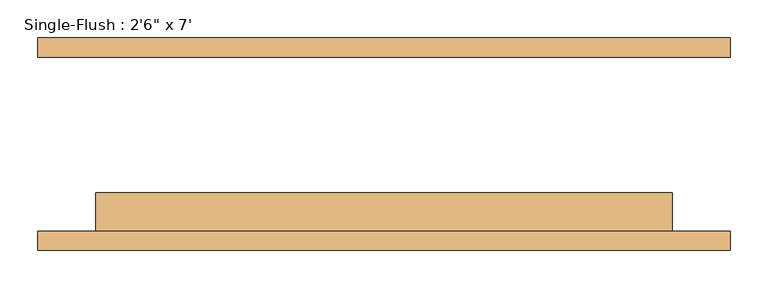
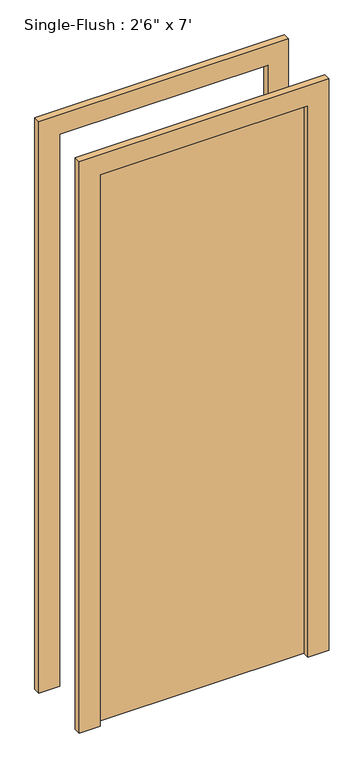
"""IFC4 building model written with IfcOpenShell, lengths in millimetres: door geometry."""

from ifc_helpers import new_model, si_unit, frame, origin, origin_with_axes, place, context, project, spatial, polyline, outline, extrude, source, transform, mapped, element, save


def door_e31f6e4d(model_context):
    return source(origin(), model_context, "Body", "SweptSolid", [
        extrude(outline(polyline([(2209.8, -457.2), (0.0, -457.2), (0.0, -381.0), (2133.6, -381.0), (2133.6, 381.0), (0.0, 381.0), (0.0, 457.2), (2209.8, 457.2), (2209.8, -457.2)])), frame((0.0, -140.4, 0.0), z_axis=(0.0, 1.0, 0.0), x_axis=(0.0, 0.0, 1.0)), (0.0, 0.0, 1.0), 25.4),
        extrude(outline(polyline([(2209.8, 457.2), (2209.8, -457.2), (0.0, -457.2), (0.0, -381.0), (2133.6, -381.0), (2133.6, 381.0), (0.0, 381.0), (0.0, 457.2), (2209.8, 457.2)])), frame((0.0, 115.0, 0.0), z_axis=(0.0, 1.0, 0.0), x_axis=(0.0, 0.0, 1.0)), (0.0, 0.0, 1.0), 25.4),
        extrude(outline(polyline([(381.0, -64.2), (381.0, -115.0), (-381.0, -115.0), (-381.0, -64.2), (381.0, -64.2)])), origin_with_axes(), (0.0, 0.0, 1.0), 2133.6),
    ])


if __name__ == "__main__":
    model = new_model("IFC4")
    model_context = context("Model", 3, world=origin())
    ifc_project = project(units=[si_unit("LENGTHUNIT", "METRE", prefix="MILLI")], contexts=[model_context])
    site = spatial("IfcSite", under=ifc_project)
    building = spatial("IfcBuilding", under=site)
    placement = place(None, origin())
    door_shape = door_e31f6e4d(model_context)
    element("IfcDoor", 1, ObjectType="Single-Flush : 2'6\" x 7'", at=placement, inside=building, context=model_context, shape_type="MappedRepresentation", body=[
        mapped(door_shape, transform((0.0, 0.0, 0.0), x_axis=(1.0, 0.0, 0.0), y_axis=(0.0, 1.0, 0.0), z_axis=(0.0, 0.0, 1.0))),
    ])
    save(model, "model.ifc")

# Revit data of these elements
# Type "Single-Flush : 2'6\" x 7'"
#   Type Mark = "10"
#   Construction Type Id = "MDOOR"
#   Assembly Code = "C1020"
#   Analytic Construction = "Metal"
#   Thickness = 0' - 2"
#   Heat Transfer Coefficient (U) = 0.651978 BTU/(h·ft²·°F)
#   Height = 7' - 0"
#   Trim Projection Ext = 0' - 1"
#   Trim Projection Int = 0' - 1"
#   Trim Width = 0' - 3"
#   Width = 2' - 6"
#   Define Thermal Properties by = 1
#   Door Material = Door - Panel
#   Frame Material = Door - Frame
#   Visual Light Transmittance = 0
#   Solar Heat Gain Coefficient = 0
#   Function = (empty or 0)
#   Wall Closure = (empty or 0)
# Element 1 (IfcDoor, "Single-Flush : 2'6\" x 7'")
#   Materials on its faces: "Door - Frame", "Door - Panel"
# Materials
#   "Door - Panel": class "Wood", colour RGB 210 159 95, transparency 0, Cost = 0
#   "Door - Frame": colour RGB 118 70 51, transparency 0, Cost = 0
